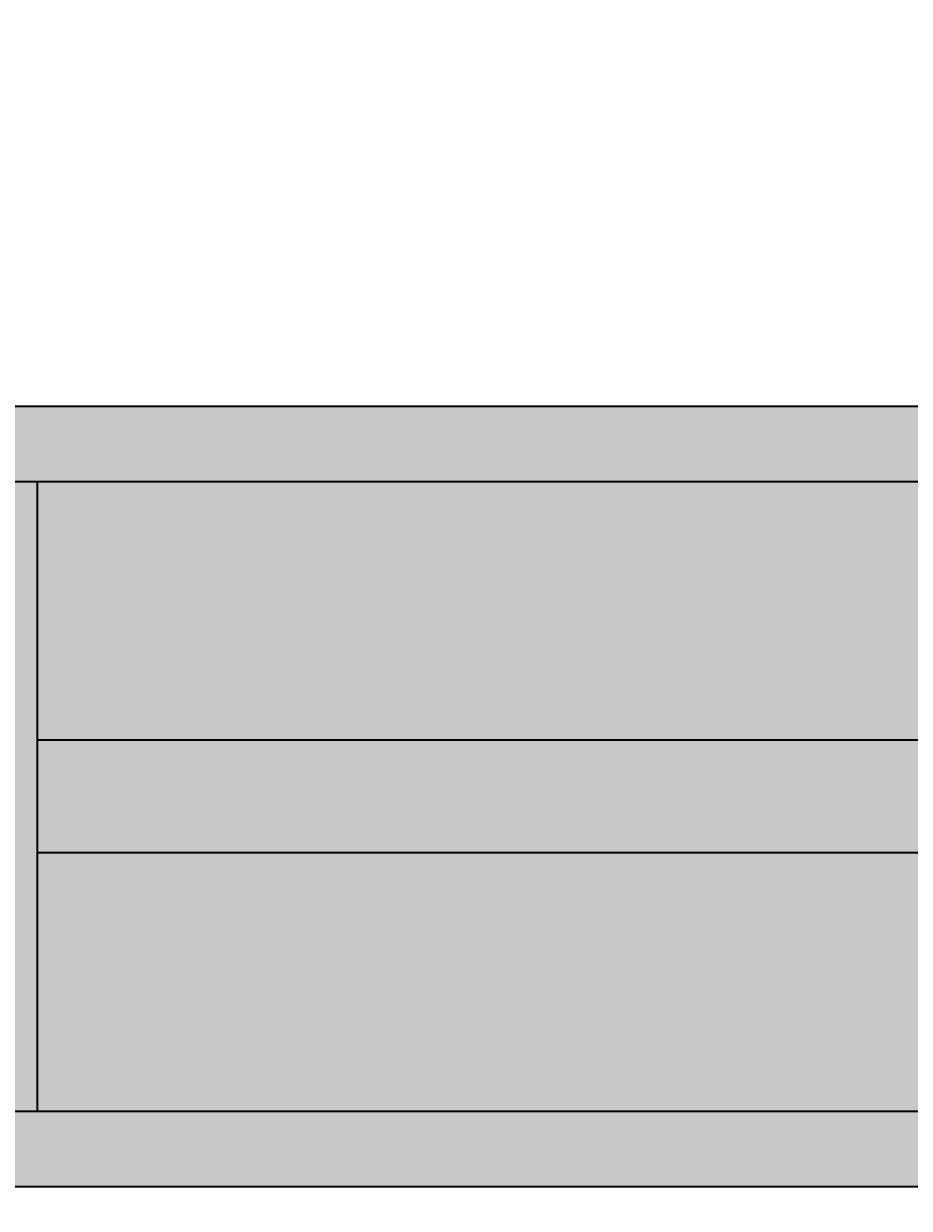
# Model space of a CAD drawing. Units: millimetres. Extents: x -11 to 280, y -4 to 208.
# Tile 27 of 55: x 163 to 186, y 22 to 54. Entities that reach past the tile are written whole.
import ezdxf

# ---------------------------------------------------------------- set-up
doc = ezdxf.new("R2010")
doc.units = ezdxf.units.MM
for name, color, linetype, lineweight in [('M-DIMS', 2, 'Continuous', 18), ('M-HYDR-CYL', 7, 'Continuous', 35), ('M-HYDR-CYL-PATT', 252, 'Continuous', 13)]:
    doc.layers.add(name, color=color, linetype=linetype, lineweight=lineweight)
doc.styles.get("Standard").update_dxf_attribs({"font": 'arial.ttf'})
doc.dimstyles.get("Standard").update_dxf_attribs({"dimtxt": 0.18, "dimasz": 0.18, "dimexe": 0.18, "dimexo": 0.0625, "dimgap": 0.09, "dimtad": 0, "dimtih": 1, "dimtoh": 1, "dimdec": 4, "dimzin": 0, "dimdsep": 46, "dimtxsty": 'Standard', "dimcen": 0.09, "dimadec": 0, "dimazin": 0, "dimtfac": 1, "dimtdec": 4, "dimtofl": 0, "dimtmove": 0, "dimatfit": 3, "dimfxl": 1, "dimtolj": 1, "dimtzin": 0, "dimarcsym": 0})

# ---------------------------------------------------------------- blocks, each defined once
blk = doc.blocks.new('*D4')
at = {"layer": 'Defpoints', "color": 0, "transparency": 16777216}
for p in [(4.763, 84.426), (266.035, 51.733), (266.035, -3.415)]:
    blk.add_point(p, dxfattribs=at)
at = {"layer": 'M-DIMS', "color": 0, "lineweight": -2, "transparency": 16777216}
for p, q in [((4.763, 84.364), (4.763, -3.595)), ((266.035, 51.67), (266.035, -3.595)), ((4.943, -3.415), (134.934, -3.415)), ((265.855, -3.415), (135.864, -3.415))]:
    blk.add_line(p, q, dxfattribs=at)
at = {"layer": 'M-DIMS', "color": 0, "transparency": 16777216}
for points in [[(4.943, -3.385), (4.943, -3.445), (4.763, -3.415)], [(265.855, -3.385), (265.855, -3.445), (266.035, -3.415)]]:
    blk.add_solid(points, dxfattribs=at)
at = {"layer": 'M-DIMS', "color": 0, "transparency": 16777216, "insert": (135.399, -3.415), "char_height": 0.18, "attachment_point": 5}
blk.add_mtext('\\A1;261.27', dxfattribs=at)
blk = doc.blocks.new('*D5')
at = {"layer": 'Defpoints', "color": 0, "transparency": 16777216}
for p in [(24.759, 192.645), (-10.087, 11.435), (261.686, 11.435)]:
    blk.add_point(p, dxfattribs=at)
at = {"layer": 'M-DIMS', "color": 0, "lineweight": -2, "transparency": 16777216}
for p, q in [((24.696, 192.645), (-10.267, 192.645)), ((-10.087, 192.465), (-10.087, 102.222)), ((-10.087, 11.615), (-10.087, 101.858)), ((261.624, 11.435), (-10.267, 11.435))]:
    blk.add_line(p, q, dxfattribs=at)
at = {"layer": 'M-DIMS', "color": 0, "transparency": 16777216}
for points in [[(-10.117, 192.465), (-10.057, 192.465), (-10.087, 192.645)], [(-10.117, 11.615), (-10.057, 11.615), (-10.087, 11.435)]]:
    blk.add_solid(points, dxfattribs=at)
at = {"layer": 'M-DIMS', "color": 0, "transparency": 16777216, "insert": (-10.087, 102.04), "char_height": 0.18, "attachment_point": 5}
blk.add_mtext('\\A1;181.2', dxfattribs=at)
blk = doc.blocks.new('*D18')
at = {"layer": 'Defpoints', "color": 0, "transparency": 16777216}
for p in [(173.804, 207.495), (173.804, 65.064), (151.022, 43.599)]:
    blk.add_point(p, dxfattribs=at)
at = {"layer": 'M-DIMS', "color": 0, "lineweight": -2, "transparency": 16777216}
for p, q in [((151.022, 43.662), (151.022, 207.675)), ((173.804, 65.126), (173.804, 207.675)), ((151.202, 207.495), (162.017, 207.495)), ((173.624, 207.495), (162.808, 207.495))]:
    blk.add_line(p, q, dxfattribs=at)
at = {"layer": 'M-DIMS', "color": 0, "transparency": 16777216}
for points in [[(151.202, 207.525), (151.202, 207.465), (151.022, 207.495)], [(173.624, 207.525), (173.624, 207.465), (173.804, 207.495)]]:
    blk.add_solid(points, dxfattribs=at)
at = {"layer": 'M-DIMS', "color": 0, "transparency": 16777216, "insert": (162.413, 207.495), "char_height": 0.18, "attachment_point": 5}
blk.add_mtext('\\A1;22.78', dxfattribs=at)
blk = doc.blocks.new('*D20')
at = {"layer": 'Defpoints', "color": 0, "transparency": 16777216}
for p in [(231.68, 207.495), (151.022, 43.599), (231.68, 43.599)]:
    blk.add_point(p, dxfattribs=at)
at = {"layer": 'M-DIMS', "color": 0, "lineweight": -2, "transparency": 16777216}
for p, q in [((151.022, 43.662), (151.022, 207.675)), ((231.68, 43.662), (231.68, 207.675)), ((151.202, 207.495), (190.957, 207.495)), ((231.5, 207.495), (191.745, 207.495))]:
    blk.add_line(p, q, dxfattribs=at)
at = {"layer": 'M-DIMS', "color": 0, "transparency": 16777216}
for points in [[(151.202, 207.525), (151.202, 207.465), (151.022, 207.495)], [(231.5, 207.525), (231.5, 207.465), (231.68, 207.495)]]:
    blk.add_solid(points, dxfattribs=at)
at = {"layer": 'M-DIMS', "color": 0, "transparency": 16777216, "insert": (191.351, 207.495), "char_height": 0.18, "attachment_point": 5}
blk.add_mtext('\\A1;80.66', dxfattribs=at)

msp = doc.modelspace()

# ---------------------------------------------------------------- hatches: boundary and pattern name
at = {"layer": 'M-HYDR-CYL-PATT'}
h = msp.add_hatch(color=256, dxfattribs=at)
h.set_gradient(color1=(128, 128, 128), color2=(99, 100, 102), tint=1)
h.paths.add_polyline_path([(163.0955, 41.5991), (160.6935, 41.5991), (160.6935, 24.846), (163.0955, 24.846)])
h.paths.add_polyline_path([(259.871, 34.7226), (163.0955, 34.7226), (163.0955, 31.7226), (259.871, 31.7226, 1)])
h.paths.add_polyline_path([(257.0171, 42.0966), (265.5958, 50.6754, 1), (263.4745, 52.7967), (253.6316, 42.9537), (253.6316, 34.7226), (257.0171, 34.7226)])
h.paths.add_polyline_path([(257.0171, 25.6028), (257.0171, 31.7226), (253.6316, 31.7226), (253.6316, 26.785), (249.6456, 22.7991), (249.6456, 13.7204, 1), (252.6456, 13.7204), (252.6456, 21.2313)])
h.paths.add_polyline_path([(265.4334, 20.9382), (261.6863, 20.9382), (261.6863, 11.4346), (265.4334, 11.4346)])
h.paths.add_polyline_path([(261.6863, 17.1598), (252.6456, 17.1598), (252.6456, 15.9126), (261.6863, 15.9126)])
h = msp.add_hatch(color=256, dxfattribs=at)
h.set_gradient(color1=(102, 52, 60), color2=(102, 52, 60), tint=1)
h.paths.add_polyline_path([(153.0217, 24.846), (153.0217, 41.5991), (156.2446, 41.5991), (156.2446, 43.5991), (151.0217, 43.5991), (151.0217, 22.846), (231.6803, 22.846), (231.6803, 31.7226), (229.6803, 31.7226), (229.6803, 24.846)])
h.paths.add_polyline_path([(159.7446, 43.5991), (159.7446, 41.5991), (163.0955, 41.5991), (229.6803, 41.5991), (229.6803, 34.7226), (231.6803, 34.7226), (231.6803, 43.5991)], flags=17)
h = msp.add_hatch(color=256, dxfattribs=at)
h.set_gradient(color1=(76, 38, 47), color2=(34, 52, 110), tint=1, name='INVCYLINDER')
h.paths.add_polyline_path([(163.0955, 41.5991), (163.0955, 34.7226), (229.6803, 34.7226), (229.6803, 41.5991)])
h.paths.add_polyline_path([(229.6803, 24.846), (229.6803, 31.7226), (163.0955, 31.7226), (163.0955, 24.846)])

# ---------------------------------------------------------------- linework, layer by layer
at = {"layer": 'M-HYDR-CYL'}
for p, q in [((259.871, 34.7226), (163.0955, 34.7226)), ((259.871, 31.7226), (163.0955, 31.7226))]:
    msp.add_line(p, q, dxfattribs=at)
for points in [[(231.6803, 31.7226), (231.6803, 22.846), (151.0217, 22.846), (151.0217, 43.5991), (156.2446, 43.5991)], [(159.7446, 43.5991), (231.6803, 43.5991), (231.6803, 34.7226)], [(229.6803, 31.7226), (229.6803, 24.846), (153.0217, 24.846), (153.0217, 41.5991), (156.2446, 41.5991)], [(159.7446, 41.5991), (163.0955, 41.5991), (163.0955, 24.846), (154.7803, 24.846)], [(159.7446, 41.5991), (229.6803, 41.5991), (229.6803, 34.7226)]]:
    msp.add_lwpolyline(points, dxfattribs=at)

# ---------------------------------------------------------------- dimensions: what is measured, and where the dimension line sits
at = {"layer": 'M-DIMS'}
for base, p1, p2, picture, middle in [((173.8038, 207.495), (151.0217, 43.5991), (173.8038, 65.0638), '*D18', (162.4127, 207.495)), ((231.6803, 207.495), (151.0217, 43.5991), (231.6803, 43.5991), '*D20', (191.351, 207.495)), ((266.0352, -3.4154), (4.7635, 84.4261), (266.0352, 51.7328), '*D4', (135.3993, -3.4154))]:
    dim = msp.add_linear_dim(base=base, p1=p1, p2=p2, dimstyle='Standard', override={"dimdec": 2, "dimlfac": 1, "dimrnd": 0, "dimzin": 0, "dimdsep": 46, "dimlunit": 2}, dxfattribs=at)
    dim.commit()
    dim.dimension.update_dxf_attribs({"geometry": picture, "text_midpoint": middle})
dim = msp.add_linear_dim(base=(-10.0865, 11.4346), p1=(24.7588, 192.645), p2=(261.6863, 11.4346), angle=90, dimstyle='Standard', override={"dimdec": 1, "dimlfac": 1, "dimrnd": 0, "dimzin": 0, "dimdsep": 46, "dimlunit": 2}, dxfattribs=at)
dim.commit()
dim.dimension.update_dxf_attribs({"geometry": '*D5', "text_midpoint": (-10.0865, 102.0398)})

doc.saveas('drawing.dxf')
